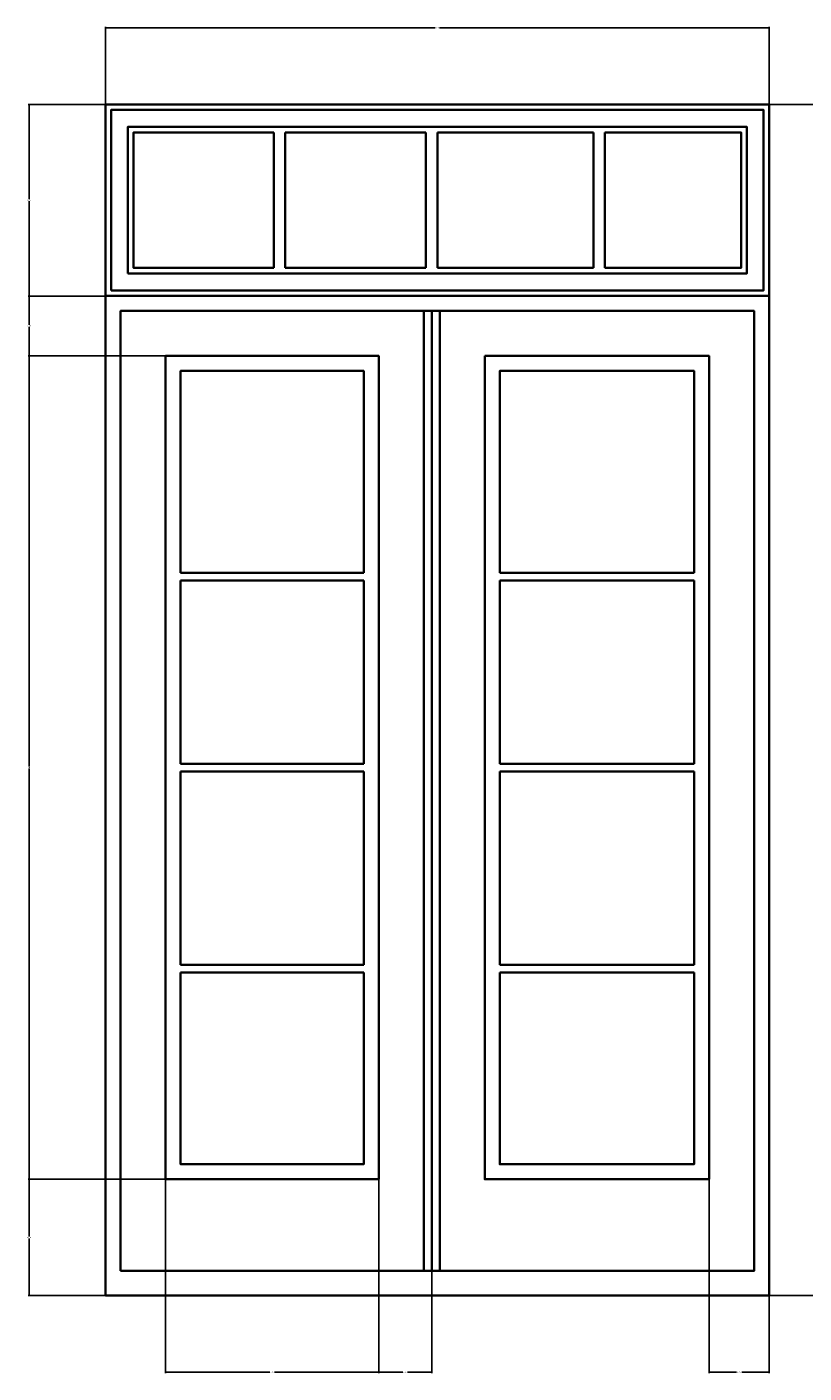
# Model space of a CAD drawing. Units: inches. Extents: x 1318 to 1980, y 617 to 1423.
# Tile 4 of 7: x 1511 to 1650, y 944 to 1184. Entities that reach past the tile are written whole.
import ezdxf

# ---------------------------------------------------------------- set-up
doc = ezdxf.new("R2010")
doc.units = ezdxf.units.IN
doc.header["$MEASUREMENT"] = 0
doc.layers.add('A-ANNO-DIMS', color=2, linetype='Continuous', lineweight=18)
doc.layers.add('A-DOOR', color=4, linetype='Continuous', lineweight=35)
doc.styles.get("Standard").update_dxf_attribs({"font": 'arial.ttf'})
doc.dimstyles.get("Standard").update_dxf_attribs({"dimtxt": 0.18, "dimasz": 0.18, "dimexe": 0.18, "dimexo": 0.0625, "dimgap": 0.09, "dimtad": 0, "dimtih": 1, "dimtoh": 1, "dimdec": 0, "dimzin": 0, "dimdsep": 46, "dimlunit": 3, "dimtxsty": 'Standard', "dimcen": 0.09, "dimadec": 0, "dimazin": 0, "dimtfac": 1, "dimtdec": 0, "dimtofl": 0, "dimtmove": 0, "dimatfit": 3, "dimfxl": 1, "dimtolj": 1, "dimtzin": 0, "dimarcsym": 0})

# ---------------------------------------------------------------- blocks, each defined once
blk = doc.blocks.new('*D48')
at = {"layer": 'A-ANNO-DIMS', "color": 0, "lineweight": -2, "transparency": 16777216}
for p, q in [((1525.23, 1170.47), (1525.23, 1184.24)), ((1525.41, 1184.06), (1584.05, 1184.06)), ((1643.45, 1184.06), (1584.82, 1184.06)), ((1643.63, 1170.47), (1643.63, 1184.24))]:
    blk.add_line(p, q, dxfattribs=at)
at = {"layer": 'A-ANNO-DIMS', "color": 0, "transparency": 16777216}
for points in [[(1525.41, 1184.09), (1525.41, 1184.03), (1525.23, 1184.06)], [(1643.45, 1184.09), (1643.45, 1184.03), (1643.63, 1184.06)]]:
    blk.add_solid(points, dxfattribs=at)
at = {"layer": 'Defpoints', "color": 0, "transparency": 16777216}
for p in [(1643.63, 1184.06), (1525.23, 1170.41), (1643.63, 1170.41)]:
    blk.add_point(p, dxfattribs=at)
at = {"layer": 'A-ANNO-DIMS', "color": 0, "transparency": 16777216, "insert": (1584.43, 1184.06), "char_height": 0.18, "attachment_point": 5}
blk.add_mtext('\\A1;118.4', dxfattribs=at)
blk = doc.blocks.new('*D49')
at = {"layer": 'A-ANNO-DIMS', "color": 0, "lineweight": -2, "transparency": 16777216}
for p, q in [((1643.69, 1170.41), (1657.46, 1170.41)), ((1657.28, 1170.23), (1657.28, 1064.23)), ((1657.28, 957.88), (1657.28, 1063.87)), ((1643.69, 957.7), (1657.46, 957.7))]:
    blk.add_line(p, q, dxfattribs=at)
at = {"layer": 'A-ANNO-DIMS', "color": 0, "transparency": 16777216}
for points in [[(1657.25, 1170.23), (1657.31, 1170.23), (1657.28, 1170.41)], [(1657.25, 957.88), (1657.31, 957.88), (1657.28, 957.7)]]:
    blk.add_solid(points, dxfattribs=at)
at = {"layer": 'Defpoints', "color": 0, "transparency": 16777216}
for p in [(1643.63, 1170.41), (1657.28, 1170.41), (1643.63, 957.7)]:
    blk.add_point(p, dxfattribs=at)
at = {"layer": 'A-ANNO-DIMS', "color": 0, "transparency": 16777216, "insert": (1657.28, 1064.05), "char_height": 0.18, "attachment_point": 5}
blk.add_mtext('\\A1;212.7', dxfattribs=at)
blk = doc.blocks.new('*D50')
at = {"layer": 'A-ANNO-DIMS', "color": 0, "lineweight": -2, "transparency": 16777216}
for p, q in [((1632.93, 978.41), (1632.93, 943.87)), ((1643.63, 957.63), (1643.63, 943.87)), ((1633.11, 944.05), (1637.82, 944.05)), ((1643.45, 944.05), (1638.74, 944.05))]:
    blk.add_line(p, q, dxfattribs=at)
at = {"layer": 'A-ANNO-DIMS', "color": 0, "transparency": 16777216}
for points in [[(1633.11, 944.08), (1633.11, 944.02), (1632.93, 944.05)], [(1643.45, 944.08), (1643.45, 944.02), (1643.63, 944.05)]]:
    blk.add_solid(points, dxfattribs=at)
at = {"layer": 'Defpoints', "color": 0, "transparency": 16777216}
for p in [(1632.93, 978.48), (1643.63, 957.7), (1643.63, 944.05)]:
    blk.add_point(p, dxfattribs=at)
at = {"layer": 'A-ANNO-DIMS', "color": 0, "transparency": 16777216, "insert": (1638.28, 944.05), "char_height": 0.18, "attachment_point": 5}
blk.add_mtext('\\A1;10.705', dxfattribs=at)
blk = doc.blocks.new('*D51')
at = {"layer": 'A-ANNO-DIMS', "color": 0, "lineweight": -2, "transparency": 16777216}
for p, q in [((1535.94, 978.41), (1535.94, 943.87)), ((1573.97, 978.41), (1573.97, 943.87)), ((1536.12, 944.05), (1554.56, 944.05)), ((1573.79, 944.05), (1555.35, 944.05))]:
    blk.add_line(p, q, dxfattribs=at)
at = {"layer": 'A-ANNO-DIMS', "color": 0, "transparency": 16777216}
for points in [[(1536.12, 944.08), (1536.12, 944.02), (1535.94, 944.05)], [(1573.79, 944.08), (1573.79, 944.02), (1573.97, 944.05)]]:
    blk.add_solid(points, dxfattribs=at)
at = {"layer": 'Defpoints', "color": 0, "transparency": 16777216}
for p in [(1535.94, 978.48), (1573.97, 978.48), (1573.97, 944.05)]:
    blk.add_point(p, dxfattribs=at)
at = {"layer": 'A-ANNO-DIMS', "color": 0, "transparency": 16777216, "insert": (1554.95, 944.05), "char_height": 0.18, "attachment_point": 5}
blk.add_mtext('\\A1;38.03', dxfattribs=at)
blk = doc.blocks.new('*D52')
at = {"layer": 'A-ANNO-DIMS', "color": 0, "lineweight": -2, "transparency": 16777216}
for p, q in [((1573.97, 978.41), (1573.97, 943.87)), ((1583.43, 962.04), (1583.43, 943.87)), ((1574.15, 944.05), (1578.3, 944.05)), ((1583.25, 944.05), (1579.09, 944.05))]:
    blk.add_line(p, q, dxfattribs=at)
at = {"layer": 'A-ANNO-DIMS', "color": 0, "transparency": 16777216}
for points in [[(1574.15, 944.08), (1574.15, 944.02), (1573.97, 944.05)], [(1583.25, 944.08), (1583.25, 944.02), (1583.43, 944.05)]]:
    blk.add_solid(points, dxfattribs=at)
at = {"layer": 'Defpoints', "color": 0, "transparency": 16777216}
for p in [(1573.97, 978.48), (1583.43, 962.1), (1583.43, 944.05)]:
    blk.add_point(p, dxfattribs=at)
at = {"layer": 'A-ANNO-DIMS', "color": 0, "transparency": 16777216, "insert": (1578.7, 944.05), "char_height": 0.18, "attachment_point": 5}
blk.add_mtext('\\A1;9.458', dxfattribs=at)
blk = doc.blocks.new('*D53')
at = {"layer": 'A-ANNO-DIMS', "color": 0, "lineweight": -2, "transparency": 16777216}
for p, q in [((1535.87, 978.48), (1511.4, 978.48)), ((1511.58, 978.3), (1511.58, 968.27)), ((1511.58, 957.88), (1511.58, 967.9)), ((1525.17, 957.7), (1511.4, 957.7))]:
    blk.add_line(p, q, dxfattribs=at)
at = {"layer": 'A-ANNO-DIMS', "color": 0, "transparency": 16777216}
for points in [[(1511.55, 978.3), (1511.61, 978.3), (1511.58, 978.48)], [(1511.55, 957.88), (1511.61, 957.88), (1511.58, 957.7)]]:
    blk.add_solid(points, dxfattribs=at)
at = {"layer": 'Defpoints', "color": 0, "transparency": 16777216}
for p in [(1511.58, 978.48), (1535.94, 978.48), (1525.23, 957.7)]:
    blk.add_point(p, dxfattribs=at)
at = {"layer": 'A-ANNO-DIMS', "color": 0, "transparency": 16777216, "insert": (1511.58, 968.09), "char_height": 0.18, "attachment_point": 5}
blk.add_mtext('\\A1;20.78', dxfattribs=at)
blk = doc.blocks.new('*D54')
at = {"layer": 'A-ANNO-DIMS', "color": 0, "lineweight": -2, "transparency": 16777216}
for p, q in [((1535.87, 1125.49), (1511.4, 1125.49)), ((1511.58, 1125.31), (1511.58, 1052.16)), ((1511.58, 978.66), (1511.58, 1051.8)), ((1535.87, 978.48), (1511.4, 978.48))]:
    blk.add_line(p, q, dxfattribs=at)
at = {"layer": 'A-ANNO-DIMS', "color": 0, "transparency": 16777216}
for points in [[(1511.55, 1125.31), (1511.61, 1125.31), (1511.58, 1125.49)], [(1511.55, 978.66), (1511.61, 978.66), (1511.58, 978.48)]]:
    blk.add_solid(points, dxfattribs=at)
at = {"layer": 'Defpoints', "color": 0, "transparency": 16777216}
for p in [(1511.58, 1125.49), (1535.94, 1125.49), (1535.94, 978.48)]:
    blk.add_point(p, dxfattribs=at)
at = {"layer": 'A-ANNO-DIMS', "color": 0, "transparency": 16777216, "insert": (1511.58, 1051.98), "char_height": 0.18, "attachment_point": 5}
blk.add_mtext('\\A1;147', dxfattribs=at)
blk = doc.blocks.new('*D55')
at = {"layer": 'A-ANNO-DIMS', "color": 0, "lineweight": -2, "transparency": 16777216}
for p, q in [((1525.17, 1136.19), (1511.4, 1136.19)), ((1511.58, 1136.01), (1511.58, 1131.02)), ((1511.58, 1125.67), (1511.58, 1130.66)), ((1535.87, 1125.49), (1511.4, 1125.49))]:
    blk.add_line(p, q, dxfattribs=at)
at = {"layer": 'A-ANNO-DIMS', "color": 0, "transparency": 16777216}
for points in [[(1511.55, 1136.01), (1511.61, 1136.01), (1511.58, 1136.19)], [(1511.55, 1125.67), (1511.61, 1125.67), (1511.58, 1125.49)]]:
    blk.add_solid(points, dxfattribs=at)
at = {"layer": 'Defpoints', "color": 0, "transparency": 16777216}
for p in [(1511.58, 1136.19), (1525.23, 1136.19), (1535.94, 1125.49)]:
    blk.add_point(p, dxfattribs=at)
at = {"layer": 'A-ANNO-DIMS', "color": 0, "transparency": 16777216, "insert": (1511.58, 1130.84), "char_height": 0.18, "attachment_point": 5}
blk.add_mtext('\\A1;10.705', dxfattribs=at)
blk = doc.blocks.new('*D56')
at = {"layer": 'A-ANNO-DIMS', "color": 0, "lineweight": -2, "transparency": 16777216}
for p, q in [((1525.17, 1170.41), (1511.4, 1170.41)), ((1511.58, 1170.23), (1511.58, 1153.48)), ((1511.58, 1136.37), (1511.58, 1153.12)), ((1525.17, 1136.19), (1511.4, 1136.19))]:
    blk.add_line(p, q, dxfattribs=at)
at = {"layer": 'A-ANNO-DIMS', "color": 0, "transparency": 16777216}
for points in [[(1511.55, 1170.23), (1511.61, 1170.23), (1511.58, 1170.41)], [(1511.55, 1136.37), (1511.61, 1136.37), (1511.58, 1136.19)]]:
    blk.add_solid(points, dxfattribs=at)
at = {"layer": 'Defpoints', "color": 0, "transparency": 16777216}
for p in [(1511.58, 1170.41), (1525.23, 1170.41), (1525.23, 1136.19)]:
    blk.add_point(p, dxfattribs=at)
at = {"layer": 'A-ANNO-DIMS', "color": 0, "transparency": 16777216, "insert": (1511.58, 1153.3), "char_height": 0.18, "attachment_point": 5}
blk.add_mtext('\\A1;34.216', dxfattribs=at)

msp = doc.modelspace()

# ---------------------------------------------------------------- linework, layer by layer
at = {"layer": 'A-DOOR'}
for p, q in [((1555.2394, 1141.1928), (1555.2394, 1165.4091)), ((1557.2655, 1141.1928), (1557.2655, 1165.4091)), ((1582.4059, 1141.1928), (1582.4059, 1165.4091)), ((1584.432, 1141.1928), (1584.432, 1165.4091)), ((1612.2958, 1141.1928), (1612.2958, 1165.4091)), ((1614.3219, 1141.1928), (1614.3219, 1165.4091)), ((1581.9964, 962.104), (1581.9964, 1133.5165)), ((1583.4254, 962.104), (1583.4254, 1133.5165)), ((1584.8545, 962.104), (1584.8545, 1133.5165)), ((1538.6132, 1086.7542), (1571.2915, 1086.7542)), ((1551.5129, 1086.7542), (1571.2915, 1086.7542)), ((1595.5593, 1086.7542), (1630.2509, 1086.7542)), ((1616.4877, 1086.7542), (1630.2509, 1086.7542)), ((1538.6132, 1085.4161), (1571.2915, 1085.4161)), ((1551.5129, 1085.4161), (1571.2915, 1085.4161)), ((1595.5593, 1085.4161), (1630.2509, 1085.4161)), ((1616.4877, 1085.4161), (1630.2509, 1085.4161)), ((1538.6132, 1052.6512), (1571.2915, 1052.6512)), ((1538.6132, 1051.3131), (1571.2915, 1051.3131)), ((1551.5129, 1052.6512), (1571.2915, 1052.6512)), ((1551.5129, 1051.3131), (1571.2915, 1051.3131)), ((1595.5593, 1052.6512), (1630.2509, 1052.6512)), ((1595.5593, 1051.3131), (1630.2509, 1051.3131)), ((1616.4877, 1052.6512), (1630.2509, 1052.6512)), ((1616.4877, 1051.3131), (1630.2509, 1051.3131)), ((1538.6132, 1016.7593), (1571.2915, 1016.7593)), ((1538.6132, 1015.4212), (1571.2915, 1015.4212)), ((1551.5129, 1016.7593), (1571.2915, 1016.7593)), ((1551.5129, 1015.4212), (1571.2915, 1015.4212)), ((1595.5593, 1016.7593), (1630.2509, 1016.7593)), ((1595.5593, 1015.4212), (1630.2509, 1015.4212)), ((1616.4877, 1016.7593), (1630.2509, 1016.7593)), ((1616.4877, 1015.4212), (1630.2509, 1015.4212))]:
    msp.add_line(p, q, dxfattribs=at)
for points in [[(1525.2321, 1136.1928), (1643.6319, 1136.1928), (1643.6319, 1170.4091), (1525.2321, 1170.4091)], [(1526.2321, 1137.1928), (1642.6319, 1137.1928), (1642.6319, 1169.4091), (1526.2321, 1169.4091)], [(1529.2321, 1140.1928), (1639.6319, 1140.1928), (1639.6319, 1166.4091), (1529.2321, 1166.4091)], [(1525.2321, 1136.1928), (1643.6319, 1136.1928), (1643.6319, 957.6972), (1525.2321, 957.6972)], [(1527.9084, 962.104), (1527.9084, 1133.5165), (1640.9557, 1133.5165), (1640.9557, 962.104)], [(1573.9677, 978.4764), (1535.937, 978.4764), (1535.937, 1125.4879), (1573.9677, 1125.4879)], [(1592.8831, 1125.4879), (1632.9271, 1125.4879), (1632.9271, 978.4764), (1592.8831, 978.4764)]]:
    msp.add_lwpolyline(points, close=True, dxfattribs=at)
for points in [[(1555.2394, 1165.4091), (1530.2321, 1165.4091), (1530.2321, 1141.1928), (1555.2394, 1141.1928)], [(1582.4059, 1165.4091), (1557.2655, 1165.4091)], [(1612.2958, 1165.4091), (1584.432, 1165.4091)], [(1614.3219, 1141.1928), (1638.6319, 1141.1928), (1638.6319, 1165.4091), (1614.3219, 1165.4091)], [(1557.2655, 1141.1928), (1582.4059, 1141.1928)], [(1584.432, 1141.1928), (1612.2958, 1141.1928)], [(1538.6132, 1086.7542), (1538.6132, 1122.8117), (1571.2915, 1122.8117), (1571.2915, 1086.7542)], [(1595.5593, 1086.7542), (1595.5593, 1122.8117), (1630.2509, 1122.8117), (1630.2509, 1086.7542)], [(1538.6132, 1052.6512), (1538.6132, 1085.4161)], [(1571.2915, 1085.4161), (1571.2915, 1052.6512)], [(1595.5593, 1052.6512), (1595.5593, 1085.4161)], [(1630.2509, 1085.4161), (1630.2509, 1052.6512)], [(1538.6132, 1016.7593), (1538.6132, 1051.3131)], [(1571.2915, 1051.3131), (1571.2915, 1016.7593)], [(1595.5593, 1016.7593), (1595.5593, 1051.3131)], [(1630.2509, 1051.3131), (1630.2509, 1016.7593)], [(1571.2915, 1015.4212), (1571.2915, 981.1526), (1538.6132, 981.1526), (1538.6132, 1015.4212)], [(1630.2509, 1015.4212), (1630.2509, 981.1526), (1595.5593, 981.1526), (1595.5593, 1015.4212)]]:
    msp.add_lwpolyline(points, dxfattribs=at)

# ---------------------------------------------------------------- dimensions: what is measured, and where the dimension line sits
at = {"layer": 'A-ANNO-DIMS'}
for base, p1, p2, override, picture, middle in [((1643.6319, 1184.0591), (1525.2321, 1170.4091), (1643.6319, 1170.4091), {"dimdec": 1, "dimlfac": 1, "dimrnd": 0, "dimzin": 0, "dimdsep": 46, "dimlunit": 2}, '*D48', (1584.432, 1184.0591)), ((1573.9677, 944.0472), (1535.937, 978.4764), (1573.9677, 978.4764), {"dimdec": 2, "dimlfac": 1, "dimrnd": 0, "dimzin": 0, "dimdsep": 46, "dimlunit": 2}, '*D51', (1554.9524, 944.0472)), ((1583.4254, 944.0472), (1573.9677, 978.4764), (1583.4254, 962.104), {"dimdec": 3, "dimlfac": 1, "dimrnd": 0, "dimzin": 0, "dimdsep": 46, "dimlunit": 2}, '*D52', (1578.6966, 944.0472)), ((1643.6319, 944.0472), (1632.9271, 978.4764), (1643.6319, 957.6972), {"dimdec": 3, "dimlfac": 1, "dimrnd": 0, "dimzin": 0, "dimdsep": 46, "dimlunit": 2}, '*D50', (1638.2795, 944.0472))]:
    dim = msp.add_linear_dim(base=base, p1=p1, p2=p2, dimstyle='Standard', override=override, dxfattribs=at)
    dim.commit()
    dim.dimension.update_dxf_attribs({"geometry": picture, "text_midpoint": middle})
for base, p1, p2, override, picture, middle in [((1511.5821, 1170.4091), (1525.2321, 1136.1928), (1525.2321, 1170.4091), {"dimdec": 3, "dimlfac": 1, "dimrnd": 0, "dimzin": 0, "dimdsep": 46, "dimlunit": 2}, '*D56', (1511.5821, 1153.3009)), ((1657.2819, 1170.4091), (1643.6319, 957.6972), (1643.6319, 1170.4091), {"dimdec": 1, "dimlfac": 1, "dimrnd": 0, "dimzin": 0, "dimdsep": 46, "dimlunit": 2}, '*D49', (1657.2819, 1064.0531)), ((1511.5821, 1136.1928), (1535.937, 1125.4879), (1525.2321, 1136.1928), {"dimdec": 3, "dimlfac": 1, "dimrnd": 0, "dimzin": 0, "dimdsep": 46, "dimlunit": 2}, '*D55', (1511.5821, 1130.8403)), ((1511.5821, 1125.4879), (1535.937, 978.4764), (1535.937, 1125.4879), {"dimdec": 0, "dimlfac": 1, "dimrnd": 0, "dimzin": 0, "dimdsep": 46, "dimlunit": 2}, '*D54', (1511.5821, 1051.9822)), ((1511.5821, 978.4764), (1525.2321, 957.6972), (1535.937, 978.4764), {"dimdec": 2, "dimlfac": 1, "dimrnd": 0, "dimzin": 0, "dimdsep": 46, "dimlunit": 2}, '*D53', (1511.5821, 968.0868))]:
    dim = msp.add_linear_dim(base=base, p1=p1, p2=p2, angle=90, dimstyle='Standard', override=override, dxfattribs=at)
    dim.commit()
    dim.dimension.update_dxf_attribs({"geometry": picture, "text_midpoint": middle})

doc.saveas('drawing.dxf')
